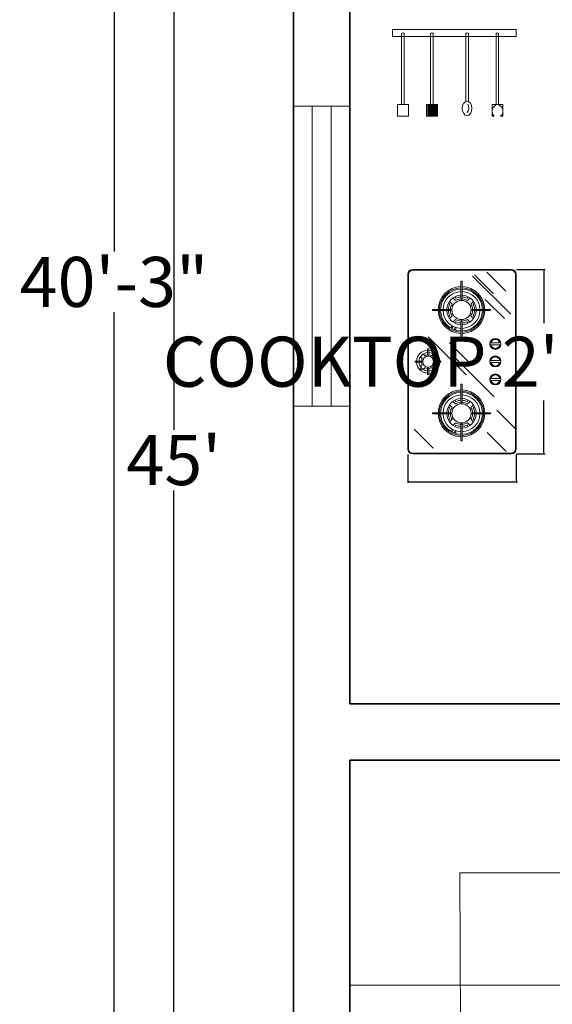
# Model space of a CAD drawing. Units: inches. Extents: x 125 to 976, y 231 to 853.
# Tile 2 of 16: x 134 to 219, y 455 to 613. Entities that reach past the tile are written whole.
import ezdxf

# ---------------------------------------------------------------- set-up
doc = ezdxf.new("R2010")
doc.units = ezdxf.units.IN
doc.header["$MEASUREMENT"] = 0
for name, color, linetype, lineweight in [('A-ANNO-DIMS', 2, 'Continuous', 18), ('A-EQPM', 8, 'Continuous', 15), ('A-FLOR-STRS', 7, 'Continuous', 18), ('A-GLAZ', 4, 'Continuous', 18), ('A-WALL', 7, 'Continuous', 35)]:
    doc.layers.add(name, color=color, linetype=linetype, lineweight=lineweight)
doc.styles.get("Standard").update_dxf_attribs({"font": 'italic8.shx'})
doc.dimstyles.get("Standard").update_dxf_attribs({"dimtxt": 8, "dimasz": 0.18, "dimexe": 0.18, "dimexo": 0.0625, "dimgap": 0.09, "dimtad": 0, "dimtih": 1, "dimtoh": 1, "dimdec": 4, "dimzin": 0, "dimdsep": 46, "dimlunit": 3, "dimtxsty": 'Standard', "dimcen": 0.09, "dimclrt": 4, "dimadec": 0, "dimazin": 0, "dimtfac": 1, "dimtdec": 4, "dimtofl": 0, "dimtmove": 0, "dimatfit": 3, "dimfxl": 1, "dimtolj": 1, "dimtzin": 0, "dimarcsym": 0})

# ---------------------------------------------------------------- blocks, each defined once
blk = doc.blocks.new('*D4')
at = {"layer": 'A-ANNO-DIMS', "color": 0, "lineweight": -2, "transparency": 16777216}
for p, q in [((177.52, 812.1), (158.26, 812.1)), ((158.44, 811.92), (158.44, 546.96)), ((158.44, 272.28), (158.44, 537.25)), ((177.52, 272.1), (158.26, 272.1))]:
    blk.add_line(p, q, dxfattribs=at)
at = {"layer": 'A-ANNO-DIMS', "color": 0, "transparency": 16777216}
for points in [[(158.41, 811.92), (158.47, 811.92), (158.44, 812.1)], [(158.41, 272.28), (158.47, 272.28), (158.44, 272.1)]]:
    blk.add_solid(points, dxfattribs=at)
at = {"layer": 'Defpoints', "color": 0, "transparency": 16777216}
for p in [(177.58, 812.1), (158.44, 272.1), (177.58, 272.1)]:
    blk.add_point(p, dxfattribs=at)
at = {"layer": 'A-ANNO-DIMS', "color": 0, "transparency": 16777216, "insert": (158.44, 542.1), "char_height": 8, "attachment_point": 5}
blk.add_mtext("\\A1;45'", dxfattribs=at)
blk = doc.blocks.new('COOKTOP-3BURNER')
for p, q in [((0, 28.74), (0, 0.79)), ((0.12, 28.74), (0.12, 0.79)), ((16.54, 29.53), (0.79, 29.53)), ((16.54, 29.41), (0.79, 29.41)), ((16.45, 22.35), (10.36, 28.44)), ((13.7, 25.61), (10.65, 28.66)), ((15.67, 26.04), (12.63, 29.08)), ((17.21, 0.79), (17.21, 28.74)), ((17.33, 0.79), (17.33, 28.74)), ((8.48, 24.8), (8.48, 27.63)), ((8.48, 27.63), (8.68, 27.63)), ((8.68, 24.8), (8.68, 27.63)), ((6.48, 24.12), (6.69, 23.92)), ((6.65, 24.4), (7.08, 23.97)), ((7.21, 24.95), (7.63, 24.53)), ((7.49, 25.12), (7.69, 24.92)), ((9.67, 25.12), (9.46, 24.92)), ((9.95, 24.95), (9.52, 24.53)), ((10.5, 24.4), (10.08, 23.97)), ((10.67, 24.12), (10.47, 23.92)), ((15.44, 21.65), (12.39, 24.7)), ((6.81, 23.13), (3.94, 23.13)), ((3.94, 23.13), (3.94, 22.93)), ((6.81, 22.93), (3.94, 22.93)), ((6.69, 22.14), (6.48, 21.94)), ((7.08, 22.09), (6.65, 21.66)), ((10.08, 22.09), (10.5, 21.66)), ((10.35, 23.13), (13.24, 23.13)), ((10.35, 22.93), (13.24, 22.93)), ((10.47, 22.14), (10.67, 21.94)), ((13.24, 23.13), (13.24, 22.93)), ((7.63, 21.53), (7.21, 21.1)), ((7.69, 21.14), (7.49, 20.93)), ((8.48, 21.26), (8.48, 18.35)), ((8.68, 21.26), (8.68, 18.35)), ((9.46, 21.14), (9.67, 20.93)), ((9.52, 21.53), (9.95, 21.1)), ((9.35, 12.64), (3.25, 18.73)), ((9.7, 14.73), (6.65, 17.78)), ((8.48, 18.35), (8.68, 18.35)), ((13.4, 17.77), (14.61, 17.77)), ((13.4, 17.46), (14.61, 17.46)), ((2.75, 15.72), (2.47, 16)), ((3.16, 16.82), (3.36, 16.82)), ((3.16, 15.84), (3.16, 16.82)), ((3.36, 15.84), (3.36, 16.82)), ((4.05, 16), (3.76, 15.72)), ((1.16, 14.86), (1.16, 14.67)), ((2.18, 14.86), (1.16, 14.86)), ((2.18, 14.67), (1.16, 14.67)), ((2.31, 15.27), (2.02, 15.56)), ((2.31, 14.26), (2.02, 13.97)), ((4.5, 15.56), (4.21, 15.27)), ((4.5, 13.97), (4.21, 14.26)), ((4.34, 14.86), (5.29, 14.86)), ((4.34, 14.67), (5.29, 14.67)), ((5.29, 14.86), (5.29, 14.67)), ((13.81, 9.14), (7.72, 15.23)), ((13.4, 14.96), (14.61, 14.96)), ((13.4, 14.65), (14.61, 14.65)), ((2.75, 13.81), (2.47, 13.53)), ((3.16, 13.69), (3.16, 12.69)), ((3.36, 12.69), (3.16, 12.69)), ((3.36, 13.69), (3.36, 12.69)), ((4.05, 13.53), (3.76, 13.81)), ((8.48, 11.18), (8.68, 11.18)), ((8.48, 8.27), (8.48, 11.18)), ((8.68, 8.27), (8.68, 11.18)), ((13.4, 12.07), (14.61, 12.07)), ((13.4, 11.76), (14.61, 11.76)), ((7.63, 8), (7.21, 8.42)), ((7.69, 8.39), (7.49, 8.59)), ((9.46, 8.39), (9.67, 8.59)), ((9.52, 8), (9.95, 8.42)), ((6.81, 6.6), (3.94, 6.6)), ((3.94, 6.4), (3.94, 6.6)), ((6.81, 6.4), (3.94, 6.4)), ((6.69, 7.39), (6.48, 7.59)), ((7.08, 7.44), (6.65, 7.87)), ((10.08, 7.44), (10.5, 7.87)), ((10.35, 6.6), (13.24, 6.6)), ((10.35, 6.4), (13.24, 6.4)), ((10.47, 7.39), (10.67, 7.59)), ((13.24, 6.4), (13.24, 6.6)), ((17.27, 3.97), (14.22, 7.02)), ((6.48, 5.41), (6.69, 5.61)), ((6.65, 5.13), (7.08, 5.56)), ((7.21, 4.57), (7.63, 5)), ((8.48, 4.93), (8.48, 2.09)), ((8.68, 4.93), (8.68, 2.09)), ((9.95, 4.57), (9.52, 5)), ((10.5, 5.13), (10.08, 5.56)), ((10.67, 5.41), (10.47, 5.61)), ((4.07, 0.94), (1.02, 3.99)), ((7.49, 4.4), (7.69, 4.61)), ((9.67, 4.4), (9.46, 4.61)), ((15.71, 0.4), (12.67, 3.44)), ((8.48, 2.09), (8.68, 2.09)), ((0.79, 0.12), (16.54, 0.12)), ((0.79, 0), (16.54, 0))]:
    blk.add_line(p, q)
for centre, radius in [((8.58, 23.03), 1.54), ((7.06, 20.26), 0.147), ((7.58, 20.04), 0.147), ((14, 17.61), 0.886), ((14, 17.61), 0.846), ((3.26, 14.76), 0.881), ((14, 14.8), 0.886), ((14, 14.8), 0.846), ((2.12, 13.62), 0.147), ((14, 11.92), 0.886), ((14, 11.92), 0.846), ((8.58, 6.5), 1.54), ((7.03, 3.73), 0.147), ((7.55, 3.51), 0.147)]:
    blk.add_circle(centre, radius)
for centre, radius, start, end in [((0.79, 28.74), 0.787, 90, 180), ((0.79, 28.74), 0.669, 90, 180), ((16.54, 28.74), 0.787, 0, 90), ((16.54, 28.74), 0.669, 0, 90), ((8.58, 23.03), 3.74, 91.5918, 178.4082), ((8.58, 23.03), 3.54, 91.5918, 178.4082), ((8.58, 23.03), 3.35, 91.6854, 178.3146), ((8.58, 23.03), 2.95, 91.9102, 178.0898), ((8.58, 23.03), 2.36, 92.388, 177.612), ((8.58, 23.03), 3.74, 1.5918, 88.4082), ((8.58, 23.03), 3.54, 1.5918, 88.4082), ((8.58, 23.03), 3.35, 1.6854, 88.3146), ((8.58, 23.03), 2.95, 1.9102, 88.0898), ((8.58, 23.03), 2.36, 2.388, 87.612), ((8.58, 23.03), 2.09, 154.8539, 177.2964), ((8.58, 23.03), 1.77, 147.8396, 176.8153), ((8.58, 23.03), 1.77, 93.1847, 122.1604), ((8.58, 23.03), 2.09, 92.7036, 115.1461), ((8.58, 24.82), 0.102, 194.2945, 345.7055), ((8.58, 23.03), 2.09, 64.8539, 87.2964), ((8.58, 23.03), 1.77, 57.8396, 86.8153), ((8.58, 23.03), 1.77, 3.1847, 32.1604), ((8.58, 23.03), 2.09, 2.7036, 25.1461), ((8.58, 23.03), 3.74, 181.5918, 268.4082), ((8.58, 23.03), 3.54, 181.5918, 268.4082), ((8.58, 23.03), 3.35, 181.6854, 268.3146), ((8.58, 23.03), 2.95, 181.9102, 268.0898), ((8.58, 23.03), 2.36, 182.388, 267.612), ((8.58, 23.03), 2.09, 182.7036, 205.1461), ((6.8, 23.03), 0.0987, 273.9579, 86.0421), ((8.58, 23.03), 1.77, 183.1847, 212.1604), ((8.58, 23.03), 2.36, 272.388, 357.612), ((8.58, 23.03), 3.54, 271.5918, 358.4082), ((8.58, 23.03), 3.35, 271.6854, 358.3146), ((8.58, 23.03), 2.95, 271.9102, 358.0898), ((8.58, 23.03), 3.74, 271.5918, 358.4082), ((8.58, 23.03), 1.77, 327.8396, 356.8153), ((10.38, 23.03), 0.103, 107.9418, 252.0582), ((8.58, 23.03), 2.09, 334.8539, 357.2964), ((8.58, 23.03), 1.77, 237.8396, 266.8153), ((8.58, 23.03), 2.09, 244.8539, 267.2964), ((8.58, 21.23), 0.104, 18.412, 161.588), ((8.58, 23.03), 1.77, 273.1847, 302.1604), ((8.58, 23.03), 2.09, 272.7036, 295.1461), ((14, 17.61), 0.728, 21.3237, 158.6763), ((13.4, 17.85), 0.0787, 158.6763, 270), ((13.4, 17.38), 0.0787, 90, 201.3237), ((14, 17.61), 0.728, 201.3237, 338.6763), ((14.61, 17.85), 0.0787, 270, 21.3237), ((14.61, 17.38), 0.0787, 338.6763, 90), ((3.26, 14.76), 1.86, 93.0255, 176.9745), ((3.26, 14.76), 1.47, 93.8363, 176.1637), ((3.26, 14.76), 1.08, 95.206, 118.0021), ((3.26, 15.85), 0.0992, 187.2236, 352.7764), ((3.26, 14.76), 1.86, 3.0255, 86.9745), ((3.26, 14.76), 1.47, 3.8363, 86.1637), ((3.26, 14.76), 1.08, 61.9979, 84.794), ((3.26, 14.76), 1.86, 183.0255, 266.9745), ((3.26, 14.76), 1.47, 183.8363, 266.1637), ((2.17, 14.76), 0.0994, 277.9505, 82.0495), ((3.26, 14.76), 1.08, 151.9979, 174.797), ((3.26, 14.76), 1.08, 185.203, 208.0021), ((3.26, 14.76), 1.86, 273.0255, 356.9745), ((3.26, 14.76), 1.47, 273.8363, 356.1637), ((3.26, 14.76), 1.08, 5.2431, 28.0021), ((3.26, 14.76), 1.08, 331.9979, 354.7569), ((4.33, 14.76), 0.0985, 88.3317, 271.6683), ((14, 14.8), 0.728, 21.3237, 158.6763), ((13.4, 15.04), 0.0787, 158.6763, 270), ((13.4, 14.57), 0.0787, 90, 201.3237), ((14, 14.8), 0.728, 201.3237, 338.6763), ((14.61, 15.04), 0.0787, 270, 21.3237), ((14.61, 14.57), 0.0787, 338.6763, 90), ((3.26, 14.76), 1.08, 241.9979, 264.8384), ((3.26, 13.66), 0.103, 17.6318, 162.3682), ((3.26, 14.76), 1.08, 275.1616, 298.0021), ((14, 11.92), 0.728, 21.3237, 158.6763), ((13.4, 12.15), 0.0787, 158.6763, 270), ((13.4, 11.68), 0.0787, 90, 201.3237), ((14, 11.92), 0.728, 201.3237, 338.6763), ((14.61, 12.15), 0.0787, 270, 21.3237), ((14.61, 11.68), 0.0787, 338.6763, 90), ((8.58, 6.5), 3.74, 91.5918, 178.4082), ((8.58, 6.5), 3.54, 91.5918, 178.4082), ((8.58, 6.5), 3.35, 91.6854, 178.3146), ((8.58, 6.5), 2.95, 91.9102, 178.0898), ((8.58, 6.5), 3.74, 1.5918, 88.4082), ((8.58, 6.5), 3.54, 1.5918, 88.4082), ((8.58, 6.5), 3.35, 1.6854, 88.3146), ((8.58, 6.5), 2.95, 1.9102, 88.0898), ((8.58, 6.5), 2.36, 92.388, 177.612), ((8.58, 6.5), 1.77, 93.1847, 122.1604), ((8.58, 6.5), 2.09, 92.7036, 115.1461), ((8.58, 8.31), 0.105, 200.5507, 339.4493), ((8.58, 6.5), 2.36, 2.388, 87.612), ((8.58, 6.5), 2.09, 64.8539, 87.2964), ((8.58, 6.5), 1.77, 57.8396, 86.8153), ((8.58, 6.5), 3.74, 181.5918, 268.4082), ((8.58, 6.5), 3.54, 181.5918, 268.4082), ((8.58, 6.5), 3.35, 181.6854, 268.3146), ((8.58, 6.5), 2.95, 181.9102, 268.0898), ((8.58, 6.5), 2.36, 182.388, 267.612), ((8.58, 6.5), 2.09, 154.8539, 177.2964), ((8.58, 6.5), 2.09, 182.7036, 205.1461), ((8.58, 6.5), 1.77, 147.8396, 176.8153), ((6.8, 6.5), 0.0991, 276.7354, 83.2646), ((8.58, 6.5), 1.77, 183.1847, 212.1604), ((8.58, 6.5), 2.95, 271.9102, 358.0898), ((8.58, 6.5), 2.36, 272.388, 357.612), ((8.58, 6.5), 3.35, 271.6854, 358.3146), ((8.58, 6.5), 3.54, 271.5918, 358.4082), ((8.58, 6.5), 3.74, 271.5918, 358.4082), ((8.58, 6.5), 1.77, 3.1847, 32.1604), ((8.58, 6.5), 1.77, 327.8396, 356.8153), ((10.39, 6.5), 0.106, 111.7885, 248.2115), ((8.58, 6.5), 2.09, 2.7036, 25.1461), ((8.58, 6.5), 2.09, 334.8539, 357.2964), ((8.58, 6.5), 1.77, 237.8396, 266.8153), ((8.58, 4.7), 0.104, 18.751, 161.249), ((8.58, 6.5), 1.77, 273.1847, 302.1604), ((8.58, 6.5), 2.09, 244.8539, 267.2964), ((8.58, 6.5), 2.09, 272.7036, 295.1461), ((0.79, 0.79), 0.787, 180, 270), ((0.79, 0.79), 0.669, 180, 270), ((16.54, 0.79), 0.669, 270, 0), ((16.54, 0.79), 0.787, 270, 0)]:
    blk.add_arc(centre, radius, start, end)
blk = doc.blocks.new('UTENSIL-RACK')
for p, q in [((0, 12.76), (0, 13.9)), ((0, 13.9), (19.77, 13.9)), ((19.77, 12.76), (0, 12.76)), ((1.43, 13.28), (1.84, 13.28)), ((1.43, 1.9), (1.43, 13.28)), ((1.84, 13.28), (1.84, 1.9)), ((6.07, 13.28), (6.49, 13.28)), ((6.07, 1.9), (6.07, 13.28)), ((6.49, 13.28), (6.49, 1.9)), ((11.72, 13.28), (12.14, 13.28)), ((11.72, 2.39), (11.72, 13.28)), ((12.14, 13.28), (12.14, 2.38)), ((16.55, 13.28), (16.96, 13.28)), ((16.55, 1.9), (16.55, 13.28)), ((16.96, 13.28), (16.96, 1.9)), ((19.77, 13.9), (19.77, 12.76)), ((0.8, 1.9), (2.53, 1.9)), ((0.8, 0), (0.8, 1.9)), ((1.84, 1.9), (1.43, 1.9)), ((2.53, 1.9), (2.53, 0)), ((5.45, 0), (5.45, 1.9)), ((5.45, 1.9), (7.18, 1.9)), ((5.66, 1.9), (5.73, 1.9)), ((5.66, 0), (5.66, 1.9)), ((5.73, 1.9), (5.73, 0)), ((5.87, 1.89), (5.94, 1.89)), ((5.87, 0), (5.87, 1.89)), ((5.94, 1.89), (5.94, 0)), ((6.49, 1.9), (6.07, 1.9)), ((6.08, 1.9), (6.16, 1.9)), ((6.08, 0), (6.08, 1.9)), ((6.16, 1.9), (6.16, 0)), ((6.29, 1.89), (6.36, 1.89)), ((6.29, 0), (6.29, 1.89)), ((6.36, 1.89), (6.36, 0)), ((6.53, 1.89), (6.6, 1.89)), ((6.53, 0), (6.53, 1.89)), ((6.6, 1.89), (6.6, 0)), ((6.75, 1.9), (6.82, 1.9)), ((6.75, 0), (6.75, 1.9)), ((6.82, 1.9), (6.82, 0.01)), ((6.95, 1.89), (7.02, 1.89)), ((6.95, 0), (6.95, 1.89)), ((7.02, 1.89), (7.02, 0)), ((7.18, 1.9), (7.18, 0)), ((15.92, 1.9), (17.65, 1.9)), ((15.92, 0), (15.92, 1.9)), ((16.96, 1.9), (16.55, 1.9)), ((17.65, 1.9), (17.65, 0)), ((2.53, 0), (0.8, 0)), ((5.45, 0), (7.18, 0)), ((5.73, 0), (5.66, 0)), ((5.94, 0), (5.87, 0)), ((6.16, 0), (6.08, 0)), ((6.36, 0), (6.29, 0)), ((6.6, 0), (6.53, 0)), ((6.82, 0.01), (6.75, 0)), ((7.18, 0), (6.8, 0)), ((7.02, 0), (6.95, 0)), ((16.26, 0.04), (15.92, 0)), ((17.65, 0), (17.27, 0))]:
    blk.add_line(p, q)
for centre, radius, start, end in [((11.03, 1.35), 1.16, 319.28, 30.314), ((16.97, 0.83), 1.06, 115.5387, 227.9153), ((16.58, 0.82), 1.07, 310.1299, 68.3923)]:
    blk.add_arc(centre, radius, start, end)
blk.add_ellipse((11.91, 1.26), major_axis=(0, 1.16), ratio=0.658977)
blk = doc.blocks.new('WINDOW-48IN')
for p, q in [((0, 0), (0, 48)), ((0, 48), (9, 48)), ((3, 0), (3, 48)), ((6, 0), (6, 48)), ((9, 48), (9, 0)), ((9, 0), (0, 0))]:
    blk.add_line(p, q)
blk = doc.blocks.new('*D50')
at = {"layer": 'A-ANNO-DIMS', "color": 0, "lineweight": -2, "transparency": 16777216}
for p, q in [((213.24, 572.61), (217.79, 572.61)), ((217.61, 572.43), (217.61, 564.03)), ((217.61, 543.26), (217.61, 551.66)), ((213.24, 543.08), (217.79, 543.08))]:
    blk.add_line(p, q, dxfattribs=at)
at = {"layer": 'A-ANNO-DIMS', "color": 0, "transparency": 16777216}
for points in [[(217.58, 572.43), (217.64, 572.43), (217.61, 572.61)], [(217.58, 543.26), (217.64, 543.26), (217.61, 543.08)]]:
    blk.add_solid(points, dxfattribs=at)
at = {"layer": 'Defpoints', "color": 0, "transparency": 16777216}
for p in [(213.18, 572.61), (217.61, 572.61), (213.18, 543.08)]:
    blk.add_point(p, dxfattribs=at)
at = {"layer": 'A-ANNO-DIMS', "color": 4, "transparency": 16777216, "insert": (217.61, 557.84), "char_height": 8, "attachment_point": 5}
blk.add_mtext('\\A1;COOKTOP 2\'-5 1/2" TYP.', dxfattribs=at)
blk = doc.blocks.new('*D51')
at = {"layer": 'A-ANNO-DIMS', "color": 0, "lineweight": -2, "transparency": 16777216}
for p, q in [((195.85, 543.02), (195.85, 538.47)), ((213.18, 543.02), (213.18, 538.47)), ((196.03, 538.65), (213, 538.65)), ((213.18, 538.65), (213.36, 538.65))]:
    blk.add_line(p, q, dxfattribs=at)
at = {"layer": 'A-ANNO-DIMS', "color": 0, "transparency": 16777216}
for points in [[(196.03, 538.68), (196.03, 538.62), (195.85, 538.65)], [(213, 538.68), (213, 538.62), (213.18, 538.65)]]:
    blk.add_solid(points, dxfattribs=at)
at = {"layer": 'Defpoints', "color": 0, "transparency": 16777216}
for p in [(195.85, 543.08), (213.18, 543.08), (213.18, 538.65)]:
    blk.add_point(p, dxfattribs=at)
at = {"layer": 'A-ANNO-DIMS', "color": 4, "transparency": 16777216, "insert": (263.35, 538.65), "char_height": 8, "attachment_point": 5}
blk.add_mtext('\\A1;1\'-5 1/2" TYP.', dxfattribs=at)
blk = doc.blocks.new('*D56')
at = {"layer": 'A-ANNO-DIMS', "color": 0, "lineweight": -2, "transparency": 16777216}
for p, q in [((177.52, 812.1), (148.7, 812.1)), ((148.88, 811.92), (148.88, 575.46)), ((148.88, 329.28), (148.88, 565.75)), ((186.52, 329.1), (148.7, 329.1))]:
    blk.add_line(p, q, dxfattribs=at)
at = {"layer": 'A-ANNO-DIMS', "color": 0, "transparency": 16777216}
for points in [[(148.85, 811.92), (148.91, 811.92), (148.88, 812.1)], [(148.85, 329.28), (148.91, 329.28), (148.88, 329.1)]]:
    blk.add_solid(points, dxfattribs=at)
at = {"layer": 'Defpoints', "color": 0, "transparency": 16777216}
for p in [(148.88, 812.1), (177.58, 812.1), (186.58, 329.1)]:
    blk.add_point(p, dxfattribs=at)
at = {"layer": 'A-ANNO-DIMS', "color": 4, "transparency": 16777216, "insert": (148.88, 570.6), "char_height": 8, "attachment_point": 5}
blk.add_mtext('\\A1;40\'-3"', dxfattribs=at)

msp = doc.modelspace()

# ---------------------------------------------------------------- linework, layer by layer
at = {"layer": 'A-FLOR-STRS'}
for p, q in [((262.5792, 476.10475), (204.18906, 476.10475)), ((204.18906, 476.10475), (204.5792, 358.10475)), ((262.5792, 458.10475), (186.5792, 458.10475))]:
    msp.add_line(p, q, dxfattribs=at)
at = {"layer": 'A-WALL'}
for p, q in [((186.5792, 614.10475), (186.5792, 503.10475)), ((186.5792, 503.10475), (267.65745, 503.10475)), ((186.5792, 494.10475), (267.65745, 494.10475)), ((186.5792, 494.10475), (186.5792, 281.10475))]:
    msp.add_line(p, q, dxfattribs=at)
msp.add_lwpolyline([(177.5792, 272.10475), (465.5792, 272.10475), (465.5792, 812.10475), (177.5792, 812.10475)], close=True, dxfattribs=at)

# ---------------------------------------------------------------- block references
at = {"layer": 'A-EQPM'}
for name, p in [('UTENSIL-RACK', (193.41, 597.09)), ('COOKTOP-3BURNER', (195.85, 543.08))]:
    msp.add_blockref(name, p, dxfattribs=at)
at = {"layer": 'A-GLAZ'}
msp.add_blockref('WINDOW-48IN', (177.57633, 550.70756), dxfattribs=at)

# ---------------------------------------------------------------- dimensions: what is measured, and where the dimension line sits
at = {"layer": 'A-ANNO-DIMS'}
for base, p1, p2, override, picture, middle in [((148.8792, 812.10475), (186.5792, 329.10475), (177.5792, 812.10475), {"dimdec": 1, "dimlfac": 1, "dimrnd": 0, "dimzin": 1, "dimdsep": 46, "dimlunit": 4, "dimfrac": 2}, '*D56', (148.8792, 570.60475)), ((158.44384, 272.10475), (177.5792, 812.10475), (177.5792, 272.10475), {"dimclrd": 0, "dimclre": 0, "dimclrt": 0}, '*D4', (158.44384, 542.10475))]:
    dim = msp.add_linear_dim(base=base, p1=p1, p2=p2, angle=90, dimstyle='Standard', override=override, dxfattribs=at)
    dim.commit()
    dim.dimension.update_dxf_attribs({"geometry": picture, "text_midpoint": middle})
dim = msp.add_linear_dim(base=(217.60518, 572.60792), p1=(213.17605, 543.08042), p2=(213.17605, 572.60792), angle=90, text='COOKTOP <> TYP.', dimstyle='Standard', override={"dimdec": 1, "dimlfac": 1, "dimrnd": 0, "dimzin": 1, "dimdsep": 46, "dimlunit": 4, "dimfrac": 2}, dxfattribs=at)
dim.commit()
dim.dimension.update_dxf_attribs({"geometry": '*D50', "text_midpoint": (217.60518, 557.84417)})
dim = msp.add_linear_dim(base=(213.17605, 538.65129), p1=(195.85325, 543.08042), p2=(213.17605, 543.08042), text='<> TYP.', dimstyle='Standard', override={"dimdec": 1, "dimlfac": 1, "dimrnd": 0, "dimzin": 1, "dimdsep": 46, "dimlunit": 4, "dimfrac": 2}, dxfattribs=at)
dim.commit()
dim.dimension.update_dxf_attribs({"geometry": '*D51', "text_midpoint": (263.35081, 538.65129)})

doc.saveas('drawing.dxf')
